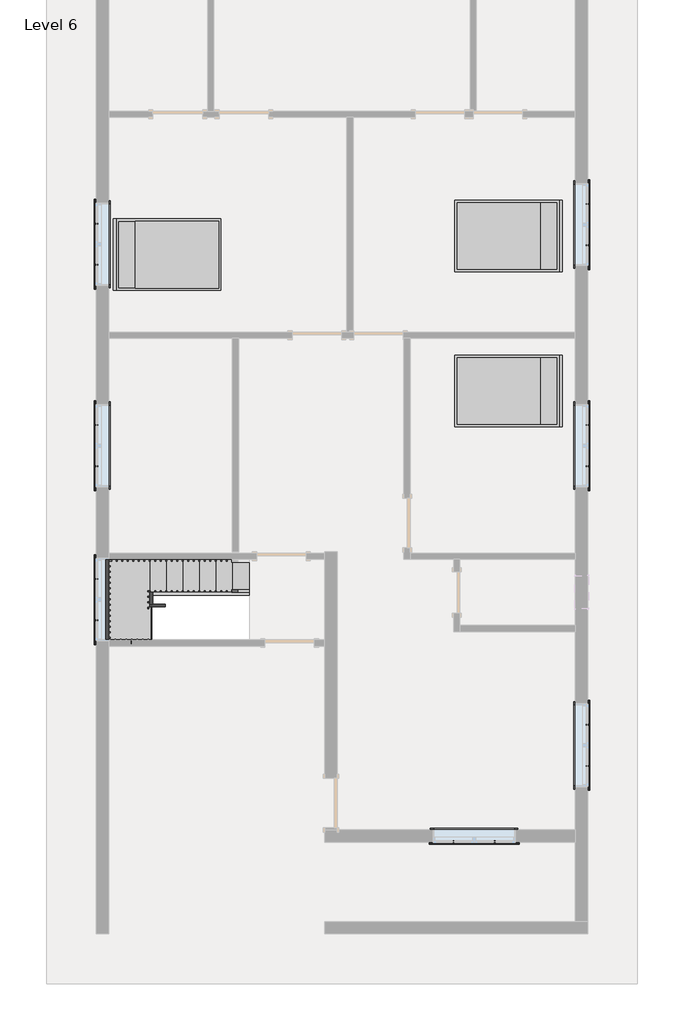
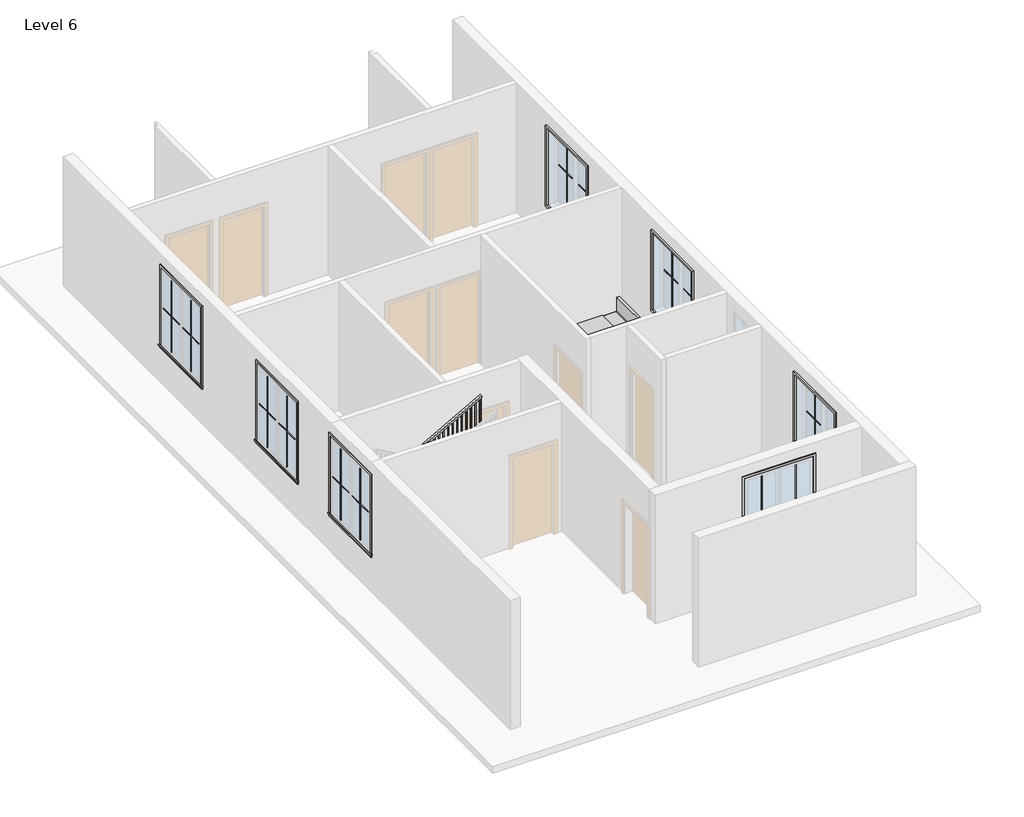
# One storey, part 3 of 3: 28 proxies, 6 members, 3 furniture elements, 1 railing, 1 stair flight.
"""IFC4 building model written with IfcOpenShell, lengths in millimetres."""

from ifc_helpers import new_model, si_unit, frame, origin, place, context, project, spatial, polyline, outline, extrude, faceted_brep, transform, mapped, element, save
from components import muntin_pattern_2x2_muntin_pattern_2x2_f6a80940, muntin_pattern_2x2_muntin_pattern_2x2_09b00a1c, trim_window_exterior_flat_with_sill_698ed857, trim_window_interior_flat_picture_frame_92551a5e, bed_17739_bed_17739_15c61121, stair_flight_411a5c89

model = new_model("IFC4")

# Units and contexts
model_context = context("Model", 3, world=origin())
ifc_project = project(units=[si_unit("LENGTHUNIT", "METRE", prefix="MILLI")], contexts=[model_context])

# Site, building, storey
site = spatial("IfcSite", under=ifc_project)
building = spatial("IfcBuilding", under=site)
storey = spatial("IfcBuildingStorey", under=building, Name="Level 6", Elevation=12801.6)

# Proxies
placement = place(None, origin())
muntin_pattern_2x2_muntin_pattern_2x2_shape = muntin_pattern_2x2_muntin_pattern_2x2_f6a80940(model_context)
element("IfcBuildingElementProxy", 1, Name="Muntin Pattern_2x2 : Muntin Pattern_2x2", ObjectType="Muntin Pattern_2x2 : Muntin Pattern_2x2", at=placement, inside=storey, context=model_context, shape_type="MappedRepresentation", body=[
    mapped(muntin_pattern_2x2_muntin_pattern_2x2_shape, transform((-5778.6870155, 3260.8309309, 13785.85), x_axis=(0.0, 1.0, 0.0), y_axis=(-1.0, 0.0, 0.0), z_axis=(0.0, 0.0, 1.0))),
])
element("IfcBuildingElementProxy", 2, Name="Muntin Pattern_2x2 : Muntin Pattern_2x2", ObjectType="Muntin Pattern_2x2 : Muntin Pattern_2x2", at=placement, inside=storey, context=model_context, shape_type="MappedRepresentation", body=[
    mapped(muntin_pattern_2x2_muntin_pattern_2x2_shape, transform((3270.0629845, 4381.6059309, 13785.85), x_axis=(0.0, -1.0, 0.0), y_axis=(1.0, 0.0, 0.0), z_axis=(0.0, 0.0, 1.0))),
])
element("IfcBuildingElementProxy", 3, Name="Muntin Pattern_2x2 : Muntin Pattern_2x2", ObjectType="Muntin Pattern_2x2 : Muntin Pattern_2x2", at=placement, inside=storey, context=model_context, shape_type="MappedRepresentation", body=[
    mapped(muntin_pattern_2x2_muntin_pattern_2x2_shape, transform((3270.0629845, 304.9059309, 13785.85), x_axis=(0.0, -1.0, 0.0), y_axis=(1.0, 0.0, 0.0), z_axis=(0.0, 0.0, 1.0))),
])
element("IfcBuildingElementProxy", 4, Name="Muntin Pattern_2x2 : Muntin Pattern_2x2", ObjectType="Muntin Pattern_2x2 : Muntin Pattern_2x2", at=placement, inside=storey, context=model_context, shape_type="MappedRepresentation", body=[
    mapped(muntin_pattern_2x2_muntin_pattern_2x2_shape, transform((3270.0629845, -5219.5940691, 13785.85), x_axis=(0.0, -1.0, 0.0), y_axis=(1.0, 0.0, 0.0), z_axis=(0.0, 0.0, 1.0))),
])
element("IfcBuildingElementProxy", 5, Name="Muntin Pattern_2x2 : Muntin Pattern_2x2", ObjectType="Muntin Pattern_2x2 : Muntin Pattern_2x2", at=placement, inside=storey, context=model_context, shape_type="MappedRepresentation", body=[
    mapped(muntin_pattern_2x2_muntin_pattern_2x2_shape, transform((1563.5004845, -7380.1815691, 13785.85), x_axis=(-1.0, 0.0, 0.0), y_axis=(0.0, -1.0, 0.0), z_axis=(0.0, 0.0, 1.0))),
])
element("IfcBuildingElementProxy", 6, Name="Muntin Pattern_2x2 : Muntin Pattern_2x2", ObjectType="Muntin Pattern_2x2 : Muntin Pattern_2x2", at=placement, inside=storey, context=model_context, shape_type="MappedRepresentation", body=[
    mapped(muntin_pattern_2x2_muntin_pattern_2x2_shape, transform((-5778.6870155, -3292.3690691, 13785.85), x_axis=(0.0, 1.0, 0.0), y_axis=(-1.0, 0.0, 0.0), z_axis=(0.0, 0.0, 1.0))),
])
element("IfcBuildingElementProxy", 7, Name="Muntin Pattern_2x2 : Muntin Pattern_2x2", ObjectType="Muntin Pattern_2x2 : Muntin Pattern_2x2", at=placement, inside=storey, context=model_context, shape_type="MappedRepresentation", body=[
    mapped(muntin_pattern_2x2_muntin_pattern_2x2_shape, transform((-5778.6870155, -453.9190691, 13785.85), x_axis=(0.0, 1.0, 0.0), y_axis=(-1.0, 0.0, 0.0), z_axis=(0.0, 0.0, 1.0))),
])
muntin_pattern_2x2_muntin_pattern_2x2_2_shape = muntin_pattern_2x2_muntin_pattern_2x2_09b00a1c(model_context)
element("IfcBuildingElementProxy", 8, Name="Muntin Pattern_2x2 : Muntin Pattern_2x2", ObjectType="Muntin Pattern_2x2 : Muntin Pattern_2x2", at=placement, inside=storey, context=model_context, shape_type="MappedRepresentation", body=[
    mapped(muntin_pattern_2x2_muntin_pattern_2x2_2_shape, transform((-5778.6870155, 4019.6559309, 13785.85), x_axis=(0.0, -1.0, 0.0), y_axis=(1.0, 0.0, 0.0), z_axis=(0.0, 0.0, 1.0))),
])
element("IfcBuildingElementProxy", 9, Name="Muntin Pattern_2x2 : Muntin Pattern_2x2", ObjectType="Muntin Pattern_2x2 : Muntin Pattern_2x2", at=placement, inside=storey, context=model_context, shape_type="MappedRepresentation", body=[
    mapped(muntin_pattern_2x2_muntin_pattern_2x2_2_shape, transform((3270.0629845, 3622.7809309, 13785.85), x_axis=(0.0, 1.0, 0.0), y_axis=(-1.0, 0.0, 0.0), z_axis=(0.0, 0.0, 1.0))),
])
element("IfcBuildingElementProxy", 10, Name="Muntin Pattern_2x2 : Muntin Pattern_2x2", ObjectType="Muntin Pattern_2x2 : Muntin Pattern_2x2", at=placement, inside=storey, context=model_context, shape_type="MappedRepresentation", body=[
    mapped(muntin_pattern_2x2_muntin_pattern_2x2_2_shape, transform((3270.0629845, -453.9190691, 13785.85), x_axis=(0.0, 1.0, 0.0), y_axis=(-1.0, 0.0, 0.0), z_axis=(0.0, 0.0, 1.0))),
])
element("IfcBuildingElementProxy", 11, Name="Muntin Pattern_2x2 : Muntin Pattern_2x2", ObjectType="Muntin Pattern_2x2 : Muntin Pattern_2x2", at=placement, inside=storey, context=model_context, shape_type="MappedRepresentation", body=[
    mapped(muntin_pattern_2x2_muntin_pattern_2x2_2_shape, transform((3270.0629845, -5978.4190691, 13785.85), x_axis=(0.0, 1.0, 0.0), y_axis=(-1.0, 0.0, 0.0), z_axis=(0.0, 0.0, 1.0))),
])
element("IfcBuildingElementProxy", 12, Name="Muntin Pattern_2x2 : Muntin Pattern_2x2", ObjectType="Muntin Pattern_2x2 : Muntin Pattern_2x2", at=placement, inside=storey, context=model_context, shape_type="MappedRepresentation", body=[
    mapped(muntin_pattern_2x2_muntin_pattern_2x2_2_shape, transform((804.6754845, -7380.1815691, 13785.85), x_axis=(1.0, 0.0, 0.0), y_axis=(0.0, 1.0, 0.0), z_axis=(0.0, 0.0, 1.0))),
])
element("IfcBuildingElementProxy", 13, Name="Muntin Pattern_2x2 : Muntin Pattern_2x2", ObjectType="Muntin Pattern_2x2 : Muntin Pattern_2x2", at=placement, inside=storey, context=model_context, shape_type="MappedRepresentation", body=[
    mapped(muntin_pattern_2x2_muntin_pattern_2x2_2_shape, transform((-5778.6870155, -2533.5440691, 13785.85), x_axis=(0.0, -1.0, 0.0), y_axis=(1.0, 0.0, 0.0), z_axis=(0.0, 0.0, 1.0))),
])
element("IfcBuildingElementProxy", 14, Name="Muntin Pattern_2x2 : Muntin Pattern_2x2", ObjectType="Muntin Pattern_2x2 : Muntin Pattern_2x2", at=placement, inside=storey, context=model_context, shape_type="MappedRepresentation", body=[
    mapped(muntin_pattern_2x2_muntin_pattern_2x2_2_shape, transform((-5778.6870155, 304.9059309, 13785.85), x_axis=(0.0, -1.0, 0.0), y_axis=(1.0, 0.0, 0.0), z_axis=(0.0, 0.0, 1.0))),
])
trim_window_exterior_flat_with_sill_shape = trim_window_exterior_flat_with_sill_698ed857(model_context)
element("IfcBuildingElementProxy", 15, Name="Trim-Window-Exterior-Flat : with Sill", ObjectType="Trim-Window-Exterior-Flat : with Sill", at=placement, inside=storey, context=model_context, shape_type="MappedRepresentation", body=[
    mapped(trim_window_exterior_flat_with_sill_shape, transform((-5788.2120155, 3640.2434309, 15544.8), x_axis=(0.0, -1.0, 0.0), y_axis=(0.0, 0.0, 1.0), z_axis=(-1.0, 0.0, 0.0))),
])
element("IfcBuildingElementProxy", 16, Name="Trim-Window-Exterior-Flat : with Sill", ObjectType="Trim-Window-Exterior-Flat : with Sill", at=placement, inside=storey, context=model_context, shape_type="MappedRepresentation", body=[
    mapped(trim_window_exterior_flat_with_sill_shape, transform((3279.5879845, 4002.1934309, 15544.8), x_axis=(0.0, 1.0, 0.0), y_axis=(0.0, 0.0, 1.0), z_axis=(1.0, 0.0, 0.0))),
])
element("IfcBuildingElementProxy", 17, Name="Trim-Window-Exterior-Flat : with Sill", ObjectType="Trim-Window-Exterior-Flat : with Sill", at=placement, inside=storey, context=model_context, shape_type="MappedRepresentation", body=[
    mapped(trim_window_exterior_flat_with_sill_shape, transform((3279.5879845, -74.5065691, 15544.8), x_axis=(0.0, 1.0, 0.0), y_axis=(0.0, 0.0, 1.0), z_axis=(1.0, 0.0, 0.0))),
])
element("IfcBuildingElementProxy", 18, Name="Trim-Window-Exterior-Flat : with Sill", ObjectType="Trim-Window-Exterior-Flat : with Sill", at=placement, inside=storey, context=model_context, shape_type="MappedRepresentation", body=[
    mapped(trim_window_exterior_flat_with_sill_shape, transform((3279.5879845, -5599.0065691, 15544.8), x_axis=(0.0, 1.0, 0.0), y_axis=(0.0, 0.0, 1.0), z_axis=(1.0, 0.0, 0.0))),
])
element("IfcBuildingElementProxy", 19, Name="Trim-Window-Exterior-Flat : with Sill", ObjectType="Trim-Window-Exterior-Flat : with Sill", at=placement, inside=storey, context=model_context, shape_type="MappedRepresentation", body=[
    mapped(trim_window_exterior_flat_with_sill_shape, transform((1184.0879845, -7389.7065691, 15544.8), x_axis=(1.0, 0.0, 0.0), y_axis=(0.0, 0.0, 1.0), z_axis=(0.0, -1.0, 0.0))),
])
element("IfcBuildingElementProxy", 20, Name="Trim-Window-Exterior-Flat : with Sill", ObjectType="Trim-Window-Exterior-Flat : with Sill", at=placement, inside=storey, context=model_context, shape_type="MappedRepresentation", body=[
    mapped(trim_window_exterior_flat_with_sill_shape, transform((-5788.2120155, -2912.9565691, 15544.8), x_axis=(0.0, -1.0, 0.0), y_axis=(0.0, 0.0, 1.0), z_axis=(-1.0, 0.0, 0.0))),
])
element("IfcBuildingElementProxy", 21, Name="Trim-Window-Exterior-Flat : with Sill", ObjectType="Trim-Window-Exterior-Flat : with Sill", at=placement, inside=storey, context=model_context, shape_type="MappedRepresentation", body=[
    mapped(trim_window_exterior_flat_with_sill_shape, transform((-5788.2120155, -74.5065691, 15544.8), x_axis=(0.0, -1.0, 0.0), y_axis=(0.0, 0.0, 1.0), z_axis=(-1.0, 0.0, 0.0))),
])
trim_window_interior_flat_picture_frame_shape = trim_window_interior_flat_picture_frame_92551a5e(model_context)
element("IfcBuildingElementProxy", 22, Name="Trim-Window-Interior-Flat : Picture Frame", ObjectType="Trim-Window-Interior-Flat : Picture Frame", at=placement, inside=storey, context=model_context, shape_type="MappedRepresentation", body=[
    mapped(trim_window_interior_flat_picture_frame_shape, transform((-5559.6120155, 3640.2434309, 15544.8), x_axis=(0.0, 1.0, 0.0), y_axis=(0.0, 0.0, 1.0), z_axis=(1.0, 0.0, 0.0))),
])
element("IfcBuildingElementProxy", 23, Name="Trim-Window-Interior-Flat : Picture Frame", ObjectType="Trim-Window-Interior-Flat : Picture Frame", at=placement, inside=storey, context=model_context, shape_type="MappedRepresentation", body=[
    mapped(trim_window_interior_flat_picture_frame_shape, transform((3050.9879845, 4002.1934309, 15544.8), x_axis=(0.0, -1.0, 0.0), y_axis=(0.0, 0.0, 1.0), z_axis=(-1.0, 0.0, 0.0))),
])
element("IfcBuildingElementProxy", 24, Name="Trim-Window-Interior-Flat : Picture Frame", ObjectType="Trim-Window-Interior-Flat : Picture Frame", at=placement, inside=storey, context=model_context, shape_type="MappedRepresentation", body=[
    mapped(trim_window_interior_flat_picture_frame_shape, transform((3050.9879845, -74.5065691, 15544.8), x_axis=(0.0, -1.0, 0.0), y_axis=(0.0, 0.0, 1.0), z_axis=(-1.0, 0.0, 0.0))),
])
element("IfcBuildingElementProxy", 25, Name="Trim-Window-Interior-Flat : Picture Frame", ObjectType="Trim-Window-Interior-Flat : Picture Frame", at=placement, inside=storey, context=model_context, shape_type="MappedRepresentation", body=[
    mapped(trim_window_interior_flat_picture_frame_shape, transform((3050.9879845, -5599.0065691, 15544.8), x_axis=(0.0, -1.0, 0.0), y_axis=(0.0, 0.0, 1.0), z_axis=(-1.0, 0.0, 0.0))),
])
element("IfcBuildingElementProxy", 26, Name="Trim-Window-Interior-Flat : Picture Frame", ObjectType="Trim-Window-Interior-Flat : Picture Frame", at=placement, inside=storey, context=model_context, shape_type="MappedRepresentation", body=[
    mapped(trim_window_interior_flat_picture_frame_shape, transform((1184.0879845, -7161.1065691, 15544.8), x_axis=(-1.0, 0.0, 0.0), y_axis=(0.0, 0.0, 1.0), z_axis=(0.0, 1.0, 0.0))),
])
element("IfcBuildingElementProxy", 27, Name="Trim-Window-Interior-Flat : Picture Frame", ObjectType="Trim-Window-Interior-Flat : Picture Frame", at=placement, inside=storey, context=model_context, shape_type="MappedRepresentation", body=[
    mapped(trim_window_interior_flat_picture_frame_shape, transform((-5559.6120155, -2912.9565691, 15544.8), x_axis=(0.0, 1.0, 0.0), y_axis=(0.0, 0.0, 1.0), z_axis=(1.0, 0.0, 0.0))),
])
element("IfcBuildingElementProxy", 28, Name="Trim-Window-Interior-Flat : Picture Frame", ObjectType="Trim-Window-Interior-Flat : Picture Frame", at=placement, inside=storey, context=model_context, shape_type="MappedRepresentation", body=[
    mapped(trim_window_interior_flat_picture_frame_shape, transform((-5559.6120155, -74.5065691, 15544.8), x_axis=(0.0, 1.0, 0.0), y_axis=(0.0, 0.0, 1.0), z_axis=(1.0, 0.0, 0.0))),
])

# Furniture
bed_17739_bed_17739_shape = bed_17739_bed_17739_15c61121(model_context)
element("IfcFurniture", 29, ObjectType="Bed_17739 : Bed_17739", at=placement, inside=storey, context=model_context, shape_type="MappedRepresentation", body=[
    mapped(bed_17739_bed_17739_shape, transform((-4454.7120155, 3449.7434309, 12801.6), x_axis=(0.0, 1.0, 0.0), y_axis=(-1.0, 0.0, 0.0), z_axis=(0.0, 0.0, 1.0))),
])
element("IfcFurniture", 30, ObjectType="Bed_17739 : Bed_17739", at=placement, inside=storey, context=model_context, shape_type="MappedRepresentation", body=[
    mapped(bed_17739_bed_17739_shape, transform((1793.6879845, 3792.6434309, 12801.6), x_axis=(0.0, -1.0, 0.0), y_axis=(1.0, 0.0, 0.0), z_axis=(0.0, 0.0, 1.0))),
])
element("IfcFurniture", 31, ObjectType="Bed_17739 : Bed_17739", at=placement, inside=storey, context=model_context, shape_type="MappedRepresentation", body=[
    mapped(bed_17739_bed_17739_shape, transform((1793.6879845, 935.1434309, 12801.6), x_axis=(0.0, -1.0, 0.0), y_axis=(1.0, 0.0, 0.0), z_axis=(0.0, 0.0, 1.0))),
])

# Members
element("IfcMember", 32, ObjectType="Stringer - 2\" Width", at=placement, inside=storey, context=model_context, shape_type="SweptSolid", body=[
    extrude(outline(polyline([(12801.6, -2968.8120155), (13009.1983948, -2968.8120155), (13996.9761726, -4746.8120155), (13648.2974984, -4746.8120155), (12801.6, -3222.7565183), (12801.6, -2968.8120155)])), frame((0.0, -2830.4065691, 0.0), z_axis=(0.0, 1.0, 0.0), x_axis=(0.0, 0.0, 1.0)), (0.0, 0.0, 1.0), 50.8),
])
element("IfcMember", 33, ObjectType="Stringer - 2\" Width", at=placement, inside=storey, context=model_context, shape_type="SweptSolid", body=[
    extrude(outline(polyline([(-4797.6120155, -2779.6065691), (-4746.8120155, -2779.6065691), (-4746.8120155, -2995.5065691), (-4797.6120155, -2995.5065691), (-4797.6120155, -2779.6065691)])), frame((0.0, 0.0, 13758.3333333), z_axis=(0.0, 0.0, 1.0), x_axis=(1.0, 0.0, 0.0)), (0.0, 0.0, 1.0), 304.8),
])
element("IfcMember", 34, ObjectType="Stringer - 2\" Width", at=placement, inside=storey, context=model_context, shape_type="SweptSolid", body=[
    extrude(outline(polyline([(14194.5317281, -4797.6120155), (13845.853054, -4797.6120155), (14861.853054, -2968.8120155), (15210.5317281, -2968.8120155), (14194.5317281, -4797.6120155)])), frame((0.0, -3046.3065691, 0.0), z_axis=(0.0, 1.0, 0.0), x_axis=(0.0, 0.0, 1.0)), (0.0, 0.0, 1.0), 50.8),
])
element("IfcMember", 35, ObjectType="Stringer - 2\" Width", at=placement, inside=storey, context=model_context, shape_type="SweptSolid", body=[
    extrude(outline(polyline([(12801.6, -2968.8120155), (13009.1983948, -2968.8120155), (14063.1333333, -4865.8949049), (14063.1333333, -5493.5165183), (12801.6, -3222.7565183), (12801.6, -2968.8120155)])), frame((0.0, -2170.0065691, 0.0), z_axis=(0.0, 1.0, 0.0), x_axis=(0.0, 0.0, 1.0)), (0.0, 0.0, 1.0), 50.8),
])
element("IfcMember", 36, ObjectType="Stringer - 2\" Width", at=placement, inside=storey, context=model_context, shape_type="SweptSolid", body=[
    extrude(outline(polyline([(-5610.4120155, -2119.2065691), (-5559.6120155, -2119.2065691), (-5559.6120155, -3674.9565691), (-5610.4120155, -3674.9565691), (-5610.4120155, -2119.2065691)])), frame((0.0, 0.0, 13758.3333333), z_axis=(0.0, 0.0, 1.0), x_axis=(1.0, 0.0, 0.0)), (0.0, 0.0, 1.0), 304.8),
])
element("IfcMember", 37, ObjectType="Stringer - 2\" Width", at=placement, inside=storey, context=model_context, shape_type="SweptSolid", body=[
    extrude(outline(polyline([(13758.3333333, -4955.1475127), (14861.853054, -2968.8120155), (15210.5317281, -2968.8120155), (13758.3333333, -5582.7691261), (13758.3333333, -4955.1475127)])), frame((0.0, -3725.7565691, 0.0), z_axis=(0.0, 1.0, 0.0), x_axis=(0.0, 0.0, 1.0)), (0.0, 0.0, 1.0), 50.8),
])

# Railing
element("IfcRailing", 38, ObjectType="Handrail - Rectangular", at=placement, inside=storey, context=model_context, shape_type="SolidModel", body=[
    faceted_brep([(-2968.8120155, -2779.6065691, 13885.3333333), (-2968.8120155, -2779.6065691, 13827.220221), (-2968.8120155, -2728.8065691, 13827.220221), (-2968.8120155, -2728.8065691, 13885.3333333), (-4721.4120155, -2779.6065691, 14859.0), (-4772.2120155, -2779.6065691, 14829.1091099), (-4772.2120155, -2728.8065691, 14829.1091099), (-4721.4120155, -2728.8065691, 14859.0), (-4721.4120155, -2779.6065691, 14901.3333333), (-4772.2120155, -2779.6065691, 14850.5333333), (-4772.2120155, -2728.8065691, 14850.5333333), (-4721.4120155, -2728.8065691, 14901.3333333), (-4797.6120155, -2779.6065691, 14901.3333333), (-4797.6120155, -2779.6065691, 14850.5333333), (-4848.4120155, -2728.8065691, 14850.5333333), (-4848.4120155, -2728.8065691, 14901.3333333), (-4797.6120155, -2855.8065691, 14901.3333333), (-4797.6120155, -2855.8065691, 14850.5333333), (-4848.4120155, -2855.8065691, 14850.5333333), (-4848.4120155, -2855.8065691, 14901.3333333), (-4797.6120155, -2970.1065691, 14901.3333333), (-4797.6120155, -3020.9065691, 14850.5333333), (-4848.4120155, -3020.9065691, 14850.5333333), (-4848.4120155, -2970.1065691, 14901.3333333), (-4797.6120155, -2970.1065691, 15113.0), (-4797.6120155, -3020.9065691, 15062.2), (-4848.4120155, -3020.9065691, 15062.2), (-4848.4120155, -2970.1065691, 15113.0), (-4797.6120155, -3046.3065691, 15113.0), (-4797.6120155, -3046.3065691, 15062.2), (-4848.4120155, -3097.1065691, 15062.2), (-4848.4120155, -3097.1065691, 15113.0), (-4721.4120155, -3046.3065691, 15113.0), (-4708.2484132, -3046.3065691, 15062.2), (-4708.2484132, -3097.1065691, 15062.2), (-4721.4120155, -3097.1065691, 15113.0), (-2968.8120155, -3046.3065691, 16086.6666667), (-2968.8120155, -3097.1065691, 16086.6666667), (-2968.8120155, -3097.1065691, 16028.5535543), (-2968.8120155, -3046.3065691, 16028.5535543)], [[[0, 1, 2, 3]], [[1, 0, 4, 5]], [[2, 1, 5, 6]], [[3, 2, 6, 7]], [[0, 3, 7, 4]], [[5, 4, 8, 9]], [[6, 5, 9, 10]], [[7, 6, 10, 11]], [[4, 7, 11, 8]], [[9, 8, 12, 13]], [[10, 9, 13, 14]], [[11, 10, 14, 15]], [[8, 11, 15, 12]], [[13, 12, 16, 17]], [[14, 13, 17, 18]], [[15, 14, 18, 19]], [[12, 15, 19, 16]], [[17, 16, 20, 21]], [[18, 17, 21, 22]], [[19, 18, 22, 23]], [[16, 19, 23, 20]], [[21, 20, 24, 25]], [[22, 21, 25, 26]], [[23, 22, 26, 27]], [[20, 23, 27, 24]], [[25, 24, 28, 29]], [[26, 25, 29, 30]], [[27, 26, 30, 31]], [[24, 27, 31, 28]], [[29, 28, 32, 33]], [[30, 29, 33, 34]], [[31, 30, 34, 35]], [[28, 31, 35, 32]], [[36, 37, 38, 39]], [[33, 32, 36, 39]], [[34, 33, 39, 38]], [[35, 34, 38, 37]], [[32, 35, 37, 36]]]),
    extrude(outline(polyline([(16009.1507765, -3003.7370155), (15002.9333333, -3003.7370155), (15002.9333333, -2984.6870155), (16019.7341099, -2984.6870155), (16009.1507765, -3003.7370155)])), frame((0.0, -3081.2315691, 0.0), z_axis=(0.0, 1.0, 0.0), x_axis=(0.0, 0.0, 1.0)), (0.0, 0.0, 1.0), 19.05),
    extrude(outline(polyline([(15952.7063321, -3105.3370155), (15002.9333333, -3105.3370155), (15002.9333333, -3086.2870155), (15963.2896654, -3086.2870155), (15952.7063321, -3105.3370155)])), frame((0.0, -3081.2315691, 0.0), z_axis=(0.0, 1.0, 0.0), x_axis=(0.0, 0.0, 1.0)), (0.0, 0.0, 1.0), 19.05),
    extrude(outline(polyline([(15896.2618876, -3206.9370155), (15002.9333333, -3206.9370155), (15002.9333333, -3187.8870155), (15906.845221, -3187.8870155), (15896.2618876, -3206.9370155)])), frame((0.0, -3081.2315691, 0.0), z_axis=(0.0, 1.0, 0.0), x_axis=(0.0, 0.0, 1.0)), (0.0, 0.0, 1.0), 19.05),
    extrude(outline(polyline([(15839.8174432, -3308.5370155), (14833.6, -3308.5370155), (14833.6, -3289.4870155), (15850.4007765, -3289.4870155), (15839.8174432, -3308.5370155)])), frame((0.0, -3081.2315691, 0.0), z_axis=(0.0, 1.0, 0.0), x_axis=(0.0, 0.0, 1.0)), (0.0, 0.0, 1.0), 19.05),
    extrude(outline(polyline([(15783.3729988, -3410.1370155), (14833.6, -3410.1370155), (14833.6, -3391.0870155), (15793.9563321, -3391.0870155), (15783.3729988, -3410.1370155)])), frame((0.0, -3081.2315691, 0.0), z_axis=(0.0, 1.0, 0.0), x_axis=(0.0, 0.0, 1.0)), (0.0, 0.0, 1.0), 19.05),
    extrude(outline(polyline([(15726.9285543, -3511.7370155), (14833.6, -3511.7370155), (14833.6, -3492.6870155), (15737.5118876, -3492.6870155), (15726.9285543, -3511.7370155)])), frame((0.0, -3081.2315691, 0.0), z_axis=(0.0, 1.0, 0.0), x_axis=(0.0, 0.0, 1.0)), (0.0, 0.0, 1.0), 19.05),
    extrude(outline(polyline([(15670.4841099, -3613.3370155), (14664.2666667, -3613.3370155), (14664.2666667, -3594.2870155), (15681.0674432, -3594.2870155), (15670.4841099, -3613.3370155)])), frame((0.0, -3081.2315691, 0.0), z_axis=(0.0, 1.0, 0.0), x_axis=(0.0, 0.0, 1.0)), (0.0, 0.0, 1.0), 19.05),
    extrude(outline(polyline([(15614.0396654, -3714.9370155), (14664.2666667, -3714.9370155), (14664.2666667, -3695.8870155), (15624.6229988, -3695.8870155), (15614.0396654, -3714.9370155)])), frame((0.0, -3081.2315691, 0.0), z_axis=(0.0, 1.0, 0.0), x_axis=(0.0, 0.0, 1.0)), (0.0, 0.0, 1.0), 19.05),
    extrude(outline(polyline([(15557.595221, -3816.5370155), (14664.2666667, -3816.5370155), (14664.2666667, -3797.4870155), (15568.1785543, -3797.4870155), (15557.595221, -3816.5370155)])), frame((0.0, -3081.2315691, 0.0), z_axis=(0.0, 1.0, 0.0), x_axis=(0.0, 0.0, 1.0)), (0.0, 0.0, 1.0), 19.05),
    extrude(outline(polyline([(15501.1507765, -3918.1370155), (14494.9333333, -3918.1370155), (14494.9333333, -3899.0870155), (15511.7341099, -3899.0870155), (15501.1507765, -3918.1370155)])), frame((0.0, -3081.2315691, 0.0), z_axis=(0.0, 1.0, 0.0), x_axis=(0.0, 0.0, 1.0)), (0.0, 0.0, 1.0), 19.05),
    extrude(outline(polyline([(15444.7063321, -4019.7370155), (14494.9333333, -4019.7370155), (14494.9333333, -4000.6870155), (15455.2896654, -4000.6870155), (15444.7063321, -4019.7370155)])), frame((0.0, -3081.2315691, 0.0), z_axis=(0.0, 1.0, 0.0), x_axis=(0.0, 0.0, 1.0)), (0.0, 0.0, 1.0), 19.05),
    extrude(outline(polyline([(15388.2618876, -4121.3370155), (14494.9333333, -4121.3370155), (14494.9333333, -4102.2870155), (15398.845221, -4102.2870155), (15388.2618876, -4121.3370155)])), frame((0.0, -3081.2315691, 0.0), z_axis=(0.0, 1.0, 0.0), x_axis=(0.0, 0.0, 1.0)), (0.0, 0.0, 1.0), 19.05),
    extrude(outline(polyline([(15331.8174432, -4222.9370155), (14325.6, -4222.9370155), (14325.6, -4203.8870155), (15342.4007765, -4203.8870155), (15331.8174432, -4222.9370155)])), frame((0.0, -3081.2315691, 0.0), z_axis=(0.0, 1.0, 0.0), x_axis=(0.0, 0.0, 1.0)), (0.0, 0.0, 1.0), 19.05),
    extrude(outline(polyline([(15275.3729988, -4324.5370155), (14325.6, -4324.5370155), (14325.6, -4305.4870155), (15285.9563321, -4305.4870155), (15275.3729988, -4324.5370155)])), frame((0.0, -3081.2315691, 0.0), z_axis=(0.0, 1.0, 0.0), x_axis=(0.0, 0.0, 1.0)), (0.0, 0.0, 1.0), 19.05),
    extrude(outline(polyline([(15218.9285543, -4426.1370155), (14325.6, -4426.1370155), (14325.6, -4407.0870155), (15229.5118876, -4407.0870155), (15218.9285543, -4426.1370155)])), frame((0.0, -3081.2315691, 0.0), z_axis=(0.0, 1.0, 0.0), x_axis=(0.0, 0.0, 1.0)), (0.0, 0.0, 1.0), 19.05),
    extrude(outline(polyline([(15162.4841099, -4527.7370155), (14156.2666667, -4527.7370155), (14156.2666667, -4508.6870155), (15173.0674432, -4508.6870155), (15162.4841099, -4527.7370155)])), frame((0.0, -3081.2315691, 0.0), z_axis=(0.0, 1.0, 0.0), x_axis=(0.0, 0.0, 1.0)), (0.0, 0.0, 1.0), 19.05),
    extrude(outline(polyline([(15106.0396654, -4629.3370155), (14156.2666667, -4629.3370155), (14156.2666667, -4610.2870155), (15116.6229988, -4610.2870155), (15106.0396654, -4629.3370155)])), frame((0.0, -3081.2315691, 0.0), z_axis=(0.0, 1.0, 0.0), x_axis=(0.0, 0.0, 1.0)), (0.0, 0.0, 1.0), 19.05),
    extrude(outline(polyline([(15049.595221, -4730.9370155), (14156.2666667, -4730.9370155), (14156.2666667, -4711.8870155), (15060.1785543, -4711.8870155), (15049.595221, -4730.9370155)])), frame((0.0, -3081.2315691, 0.0), z_axis=(0.0, 1.0, 0.0), x_axis=(0.0, 0.0, 1.0)), (0.0, 0.0, 1.0), 19.05),
    extrude(outline(polyline([(-4813.4870155, -3049.4815691), (-4813.4870155, -3068.5315691), (-4832.5370155, -3068.5315691), (-4832.5370155, -3049.4815691), (-4813.4870155, -3049.4815691)])), frame((0.0, 0.0, 13986.9333333), z_axis=(0.0, 0.0, 1.0), x_axis=(1.0, 0.0, 0.0)), (0.0, 0.0, 1.0), 1075.2666667),
    extrude(outline(polyline([(-4813.4870155, -2947.8815691), (-4813.4870155, -2966.9315691), (-4832.5370155, -2966.9315691), (-4832.5370155, -2947.8815691), (-4813.4870155, -2947.8815691)])), frame((0.0, 0.0, 13986.9333333), z_axis=(0.0, 0.0, 1.0), x_axis=(1.0, 0.0, 0.0)), (0.0, 0.0, 1.0), 863.6),
    extrude(outline(polyline([(-4813.4870155, -2846.2815691), (-4813.4870155, -2865.3315691), (-4832.5370155, -2865.3315691), (-4832.5370155, -2846.2815691), (-4813.4870155, -2846.2815691)])), frame((0.0, 0.0, 13986.9333333), z_axis=(0.0, 0.0, 1.0), x_axis=(1.0, 0.0, 0.0)), (0.0, 0.0, 1.0), 863.6),
    extrude(outline(polyline([(-4788.0870155, -2763.7315691), (-4807.1370155, -2763.7315691), (-4807.1370155, -2744.6815691), (-4788.0870155, -2744.6815691), (-4788.0870155, -2763.7315691)])), frame((0.0, 0.0, 13986.9333333), z_axis=(0.0, 0.0, 1.0), x_axis=(1.0, 0.0, 0.0)), (0.0, 0.0, 1.0), 863.6),
    extrude(outline(polyline([(14792.0674432, -4705.5370155), (13817.6, -4705.5370155), (13817.6, -4686.4870155), (14781.4841099, -4686.4870155), (14792.0674432, -4705.5370155)])), frame((0.0, -2763.7315691, 0.0), z_axis=(0.0, 1.0, 0.0), x_axis=(0.0, 0.0, 1.0)), (0.0, 0.0, 1.0), 19.05),
    extrude(outline(polyline([(14735.6229988, -4603.9370155), (13817.6, -4603.9370155), (13817.6, -4584.8870155), (14725.0396654, -4584.8870155), (14735.6229988, -4603.9370155)])), frame((0.0, -2763.7315691, 0.0), z_axis=(0.0, 1.0, 0.0), x_axis=(0.0, 0.0, 1.0)), (0.0, 0.0, 1.0), 19.05),
    extrude(outline(polyline([(14679.1785543, -4502.3370155), (13817.6, -4502.3370155), (13817.6, -4483.2870155), (14668.595221, -4483.2870155), (14679.1785543, -4502.3370155)])), frame((0.0, -2763.7315691, 0.0), z_axis=(0.0, 1.0, 0.0), x_axis=(0.0, 0.0, 1.0)), (0.0, 0.0, 1.0), 19.05),
    extrude(outline(polyline([(14622.7341099, -4400.7370155), (13648.2666667, -4400.7370155), (13648.2666667, -4381.6870155), (14612.1507765, -4381.6870155), (14622.7341099, -4400.7370155)])), frame((0.0, -2763.7315691, 0.0), z_axis=(0.0, 1.0, 0.0), x_axis=(0.0, 0.0, 1.0)), (0.0, 0.0, 1.0), 19.05),
    extrude(outline(polyline([(14566.2896654, -4299.1370155), (13648.2666667, -4299.1370155), (13648.2666667, -4280.0870155), (14555.7063321, -4280.0870155), (14566.2896654, -4299.1370155)])), frame((0.0, -2763.7315691, 0.0), z_axis=(0.0, 1.0, 0.0), x_axis=(0.0, 0.0, 1.0)), (0.0, 0.0, 1.0), 19.05),
    extrude(outline(polyline([(14509.845221, -4197.5370155), (13648.2666667, -4197.5370155), (13648.2666667, -4178.4870155), (14499.2618876, -4178.4870155), (14509.845221, -4197.5370155)])), frame((0.0, -2763.7315691, 0.0), z_axis=(0.0, 1.0, 0.0), x_axis=(0.0, 0.0, 1.0)), (0.0, 0.0, 1.0), 19.05),
    extrude(outline(polyline([(14453.4007765, -4095.9370155), (13478.9333333, -4095.9370155), (13478.9333333, -4076.8870155), (14442.8174432, -4076.8870155), (14453.4007765, -4095.9370155)])), frame((0.0, -2763.7315691, 0.0), z_axis=(0.0, 1.0, 0.0), x_axis=(0.0, 0.0, 1.0)), (0.0, 0.0, 1.0), 19.05),
    extrude(outline(polyline([(14396.9563321, -3994.3370155), (13478.9333333, -3994.3370155), (13478.9333333, -3975.2870155), (14386.3729988, -3975.2870155), (14396.9563321, -3994.3370155)])), frame((0.0, -2763.7315691, 0.0), z_axis=(0.0, 1.0, 0.0), x_axis=(0.0, 0.0, 1.0)), (0.0, 0.0, 1.0), 19.05),
    extrude(outline(polyline([(14340.5118876, -3892.7370155), (13478.9333333, -3892.7370155), (13478.9333333, -3873.6870155), (14329.9285543, -3873.6870155), (14340.5118876, -3892.7370155)])), frame((0.0, -2763.7315691, 0.0), z_axis=(0.0, 1.0, 0.0), x_axis=(0.0, 0.0, 1.0)), (0.0, 0.0, 1.0), 19.05),
    extrude(outline(polyline([(14284.0674432, -3791.1370155), (13309.6, -3791.1370155), (13309.6, -3772.0870155), (14273.4841099, -3772.0870155), (14284.0674432, -3791.1370155)])), frame((0.0, -2763.7315691, 0.0), z_axis=(0.0, 1.0, 0.0), x_axis=(0.0, 0.0, 1.0)), (0.0, 0.0, 1.0), 19.05),
    extrude(outline(polyline([(14227.6229988, -3689.5370155), (13309.6, -3689.5370155), (13309.6, -3670.4870155), (14217.0396654, -3670.4870155), (14227.6229988, -3689.5370155)])), frame((0.0, -2763.7315691, 0.0), z_axis=(0.0, 1.0, 0.0), x_axis=(0.0, 0.0, 1.0)), (0.0, 0.0, 1.0), 19.05),
    extrude(outline(polyline([(14171.1785543, -3587.9370155), (13309.6, -3587.9370155), (13309.6, -3568.8870155), (14160.595221, -3568.8870155), (14171.1785543, -3587.9370155)])), frame((0.0, -2763.7315691, 0.0), z_axis=(0.0, 1.0, 0.0), x_axis=(0.0, 0.0, 1.0)), (0.0, 0.0, 1.0), 19.05),
    extrude(outline(polyline([(14114.7341099, -3486.3370155), (13140.2666667, -3486.3370155), (13140.2666667, -3467.2870155), (14104.1507765, -3467.2870155), (14114.7341099, -3486.3370155)])), frame((0.0, -2763.7315691, 0.0), z_axis=(0.0, 1.0, 0.0), x_axis=(0.0, 0.0, 1.0)), (0.0, 0.0, 1.0), 19.05),
    extrude(outline(polyline([(14058.2896654, -3384.7370155), (13140.2666667, -3384.7370155), (13140.2666667, -3365.6870155), (14047.7063321, -3365.6870155), (14058.2896654, -3384.7370155)])), frame((0.0, -2763.7315691, 0.0), z_axis=(0.0, 1.0, 0.0), x_axis=(0.0, 0.0, 1.0)), (0.0, 0.0, 1.0), 19.05),
    extrude(outline(polyline([(14001.845221, -3283.1370155), (13140.2666667, -3283.1370155), (13140.2666667, -3264.0870155), (13991.2618876, -3264.0870155), (14001.845221, -3283.1370155)])), frame((0.0, -2763.7315691, 0.0), z_axis=(0.0, 1.0, 0.0), x_axis=(0.0, 0.0, 1.0)), (0.0, 0.0, 1.0), 19.05),
    extrude(outline(polyline([(13945.4007765, -3181.5370155), (12970.9333333, -3181.5370155), (12970.9333333, -3162.4870155), (13934.8174432, -3162.4870155), (13945.4007765, -3181.5370155)])), frame((0.0, -2763.7315691, 0.0), z_axis=(0.0, 1.0, 0.0), x_axis=(0.0, 0.0, 1.0)), (0.0, 0.0, 1.0), 19.05),
    extrude(outline(polyline([(13888.9563321, -3079.9370155), (12970.9333333, -3079.9370155), (12970.9333333, -3060.8870155), (13878.3729988, -3060.8870155), (13888.9563321, -3079.9370155)])), frame((0.0, -2763.7315691, 0.0), z_axis=(0.0, 1.0, 0.0), x_axis=(0.0, 0.0, 1.0)), (0.0, 0.0, 1.0), 19.05),
    extrude(outline(polyline([(-4813.4870155, -3062.1815691), (-4813.4870155, -3081.2315691), (-4832.5370155, -3081.2315691), (-4832.5370155, -3062.1815691), (-4813.4870155, -3062.1815691)])), frame((0.0, 0.0, 13986.9333333), z_axis=(0.0, 0.0, 1.0), x_axis=(1.0, 0.0, 0.0)), (0.0, 0.0, 1.0), 1075.2666667),
    extrude(outline(polyline([(-4813.4870155, -2763.7315691), (-4832.5370155, -2763.7315691), (-4832.5370155, -2744.6815691), (-4813.4870155, -2744.6815691), (-4813.4870155, -2763.7315691)])), frame((0.0, 0.0, 13986.9333333), z_axis=(0.0, 0.0, 1.0), x_axis=(1.0, 0.0, 0.0)), (0.0, 0.0, 1.0), 863.6),
    extrude(outline(polyline([(16017.970221, -2987.8620155), (15002.9333333, -2987.8620155), (15002.9333333, -2968.8120155), (16028.5535543, -2968.8120155), (16017.970221, -2987.8620155)])), frame((0.0, -3081.2315691, 0.0), z_axis=(0.0, 1.0, 0.0), x_axis=(0.0, 0.0, 1.0)), (0.0, 0.0, 1.0), 19.05),
    extrude(outline(polyline([(13837.8035543, -2987.8620155), (12970.9333333, -2987.8620155), (12970.9333333, -2968.8120155), (13827.220221, -2968.8120155), (13837.8035543, -2987.8620155)])), frame((0.0, -2763.7315691, 0.0), z_axis=(0.0, 1.0, 0.0), x_axis=(0.0, 0.0, 1.0)), (0.0, 0.0, 1.0), 19.05),
])

# Stair flight
stair_flight_shape = stair_flight_411a5c89(model_context)
element("IfcStairFlight", 39, ObjectType="2\" Tread 1\" Nosing 1/4\" Riser", at=placement, inside=storey, context=model_context, shape_type="MappedRepresentation", body=[
    mapped(stair_flight_shape, transform((0.0, 0.0, 0.0), x_axis=(1.0, 0.0, 0.0), y_axis=(0.0, 1.0, 0.0), z_axis=(0.0, 0.0, 1.0))),
])

save(model, "model.ifc")

# Revit data of these elements
# Type "Muntin Pattern_2x2 : Muntin Pattern_2x2"
#   Width [instance default] = 4' - 0"
#   Thickness = 0' - 0 1/2"
#   Height [instance default] = 4' - 0"
#   Distance = 0' - 0 3/4"
#   Interior Material [instance default] = none
#   Exterior Material [instance default] = none
#   Default Elevation = 0
# Type "Trim-Window-Exterior-Flat : with Sill"
#   Trim Width = 0' - 2 1/4"
#   Trim Thickness_Picture Frame = 0' - 1 1/4"
#   Trim Thickness_with Sill = 0' - 0 3/4"
#   Sill Thickness = 0' - 1 1/4"
#   Opening Width [instance default] = 2' - 0"
#   Opening Height [instance default] = 3' - 0"
#   Default Elevation = 4' - 0"
#   Sill = yes
#   Picture Frame = no
#   Trim Material [instance default] = none
# Type "Trim-Window-Interior-Flat : Picture Frame"
#   Trim Thickness_Picture Frame = 0' - 1 1/4"
#   Trim Width = 0' - 2 1/4"
#   Trim Thickness_with Sill = 0' - 0 3/4"
#   Sill Thickness = 0' - 1 1/4"
#   Opening Width [instance default] = 2' - 0"
#   Opening Height [instance default] = 3' - 0"
#   Default Elevation = 4' - 0"
#   Sill = no
#   Picture Frame = yes
#   Trim Material [instance default] = none
# Type "Bed_17739 : Bed_17739"
#   Default Elevation = 0
# Type "Handrail - Rectangular"
#   Assembly Code = "C2010400"
#   built-in parameter 1008612 = 0.0416667 (stored number, unit not read)
#   built-in parameter 1008611 = 0.0416667 (stored number, unit not read)
#   built-in parameter 1008609 = 0.333333 (stored number, unit not read)
#   built-in parameter 1008604 = 0.166667 (stored number, unit not read)
#   built-in parameter 1008603 = 0.166667 (stored number, unit not read)
#   Railing Height = 3' - 0"
#   built-in parameter 1008630 = 2
#   built-in parameter 1008610 = 2
#   built-in parameter 1008618 = Baluster - Square : 3/4"
# Elements 1, 2, 3, 4, 5, 6, 7, 8, 9, 10, 11, 12, 13, 14 (IfcBuildingElementProxy, "Muntin Pattern_2x2 : Muntin Pattern_2x2")
#   Width = 2' - 0 5/8"
#   Height = 5' - 6 1/2"
#   Interior Material = Wood - Stained
#   Exterior Material = Clad - White
#   Phase Created = New Construction
#   Materials on its faces: "Clad - White", "Wood - Stained"
# Elements 15, 16, 17, 18, 19, 20, 21 (IfcBuildingElementProxy, "Trim-Window-Exterior-Flat : with Sill")
#   Opening Width = 5' - 0"
#   Opening Height = 6' - 0"
#   Trim Material = Clad - White
#   Phase Created = New Construction
#   Materials on its faces: "Clad - White"
# Elements 22, 23, 24, 25, 26, 27, 28 (IfcBuildingElementProxy, "Trim-Window-Interior-Flat : Picture Frame")
#   Opening Width = 5' - 0"
#   Opening Height = 6' - 0"
#   Trim Material = Wood - Stained
#   Phase Created = New Construction
#   Materials on its faces: "Wood - Stained"
# Elements 29, 30, 31 (IfcFurniture, "Bed_17739 : Bed_17739")
#   Phase Created = New Construction
#   Materials on its faces: "legs", "sheets", "bed frame", "Blanket"
# Elements 32, 33, 34, 35, 36, 37 (IfcMember, "Stringer - 2\" Width")
#   Phase Created = New Construction
# Element 38 (IfcRailing, "Handrail - Rectangular")
#   Phase Created = New Construction
# Element 39 (IfcStairFlight, "2\" Tread 1\" Nosing 1/4\" Riser")
#   Phase Created = New Construction
# Materials
#   "Clad - White": class "Wood", colour RGB 242 242 238, transparency 0, Cost = 0
#   "Wood - Stained": class "Wood", colour RGB 224 178 126, transparency 0, Cost = 0
#   "legs": colour RGB 90 73 37, transparency 0, Cost = 0
#   "sheets": colour RGB 200 195 176, transparency 0, Cost = 0
#   "bed frame": colour RGB 90 73 37, transparency 0, Cost = 0
#   "Blanket": class "System", colour RGB 59 0 1, transparency 0, Cost = 0
